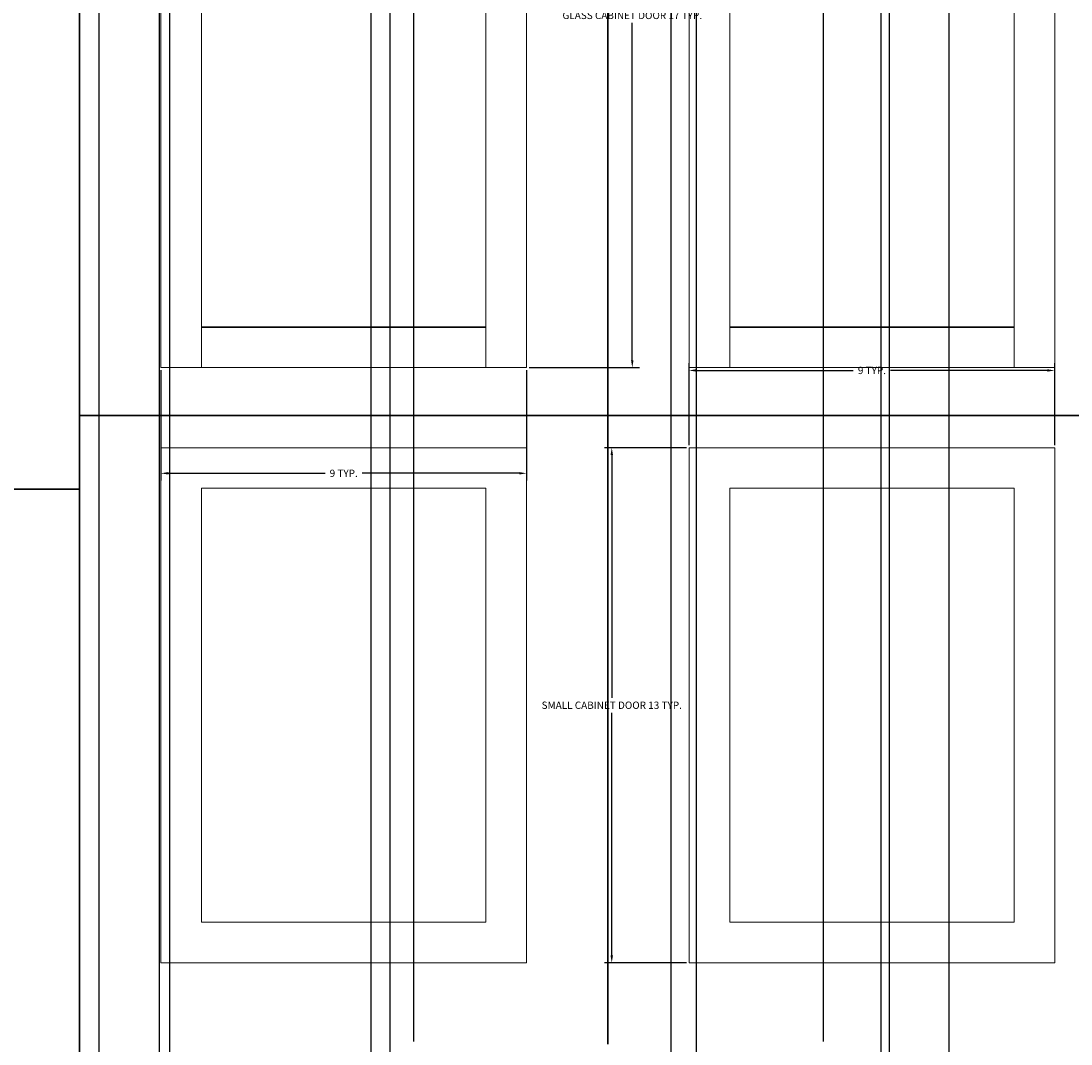
# Model space of a CAD drawing. Units: inches. Extents: x 27 to 200, y -50 to 102.
# Tile 19 of 26: x 119 to 145, y 52 to 77. Entities that reach past the tile are written whole.
import ezdxf

# ---------------------------------------------------------------- set-up
doc = ezdxf.new("R2010")
doc.units = ezdxf.units.IN
doc.header["$MEASUREMENT"] = 0
for name, color, linetype, lineweight in [('A-ANNO-DIMS', 2, 'Continuous', 18), ('A-ELEV', 7, 'Continuous', 35), ('A-FURN', 8, 'Continuous', 18)]:
    doc.layers.add(name, color=color, linetype=linetype, lineweight=lineweight)
doc.styles.get("Standard").update_dxf_attribs({"font": 'arial.ttf'})
doc.dimstyles.get("Standard").update_dxf_attribs({"dimtxt": 0.18, "dimasz": 0.18, "dimexe": 0.18, "dimexo": 0.0625, "dimgap": 0.09, "dimtad": 0, "dimtih": 1, "dimtoh": 1, "dimdec": 4, "dimzin": 0, "dimdsep": 46, "dimtxsty": 'Standard', "dimcen": 0.09, "dimadec": 0, "dimazin": 0, "dimtfac": 1, "dimtdec": 4, "dimtofl": 0, "dimtmove": 0, "dimatfit": 3, "dimfxl": 1, "dimtolj": 1, "dimtzin": 0, "dimarcsym": 0})

# ---------------------------------------------------------------- blocks, each defined once
blk = doc.blocks.new('CAB-DOOR-GLASS')
for p, q in [((0, 17.345), (9, 17.345)), ((0, 0), (0, 17.345)), ((9, 17.345), (9, 0)), ((1, 16.345), (8, 16.345)), ((1, 0), (1, 16.345)), ((8, 16.345), (8, 0)), ((9, 0), (0, 0))]:
    blk.add_line(p, q)
blk = doc.blocks.new('CAB-DOOR-SMALL')
for p, q in [((0, 0), (0, 12.683)), ((0, 12.683), (9, 12.683)), ((9, 12.683), (9, 0)), ((1, 1), (1, 11.683)), ((1, 11.683), (8, 11.683)), ((8, 11.683), (8, 1)), ((8, 1), (1, 1)), ((9, 0), (0, 0))]:
    blk.add_line(p, q)
blk = doc.blocks.new('*D9')
at = {"layer": 'A-ANNO-DIMS', "color": 0, "lineweight": -2, "transparency": 16777216}
for p, q in [((131.479, 85.926), (134.199, 85.926)), ((134.019, 85.746), (134.019, 77.437)), ((134.019, 68.761), (134.019, 77.071)), ((131.479, 68.581), (134.199, 68.581))]:
    blk.add_line(p, q, dxfattribs=at)
at = {"layer": 'A-ANNO-DIMS', "color": 0, "transparency": 16777216}
for points in [[(133.989, 85.746), (134.049, 85.746), (134.019, 85.926)], [(133.989, 68.761), (134.049, 68.761), (134.019, 68.581)]]:
    blk.add_solid(points, dxfattribs=at)
at = {"layer": 'Defpoints', "color": 0, "transparency": 16777216}
for p in [(131.417, 85.926), (134.019, 85.926), (131.417, 68.581)]:
    blk.add_point(p, dxfattribs=at)
at = {"layer": 'A-ANNO-DIMS', "color": 0, "transparency": 16777216, "insert": (134.019, 77.254), "char_height": 0.18, "attachment_point": 5}
blk.add_mtext('\\A1;GLASS CABINET DOOR 17 TYP.', dxfattribs=at)
blk = doc.blocks.new('*D10')
at = {"layer": 'A-ANNO-DIMS', "color": 0, "lineweight": -2, "transparency": 16777216}
for p, q in [((122.417, 68.519), (122.417, 65.799)), ((131.417, 68.519), (131.417, 65.799)), ((122.597, 65.979), (126.459, 65.979)), ((131.237, 65.979), (127.375, 65.979))]:
    blk.add_line(p, q, dxfattribs=at)
at = {"layer": 'A-ANNO-DIMS', "color": 0, "transparency": 16777216}
for points in [[(122.597, 66.009), (122.597, 65.949), (122.417, 65.979)], [(131.237, 66.009), (131.237, 65.949), (131.417, 65.979)]]:
    blk.add_solid(points, dxfattribs=at)
at = {"layer": 'Defpoints', "color": 0, "transparency": 16777216}
for p in [(122.417, 68.581), (131.417, 68.581), (131.417, 65.979)]:
    blk.add_point(p, dxfattribs=at)
at = {"layer": 'A-ANNO-DIMS', "color": 0, "transparency": 16777216, "insert": (126.917, 65.979), "char_height": 0.18, "attachment_point": 5}
blk.add_mtext('\\A1;9 TYP.', dxfattribs=at)
blk = doc.blocks.new('*D11')
at = {"layer": 'A-ANNO-DIMS', "color": 0, "lineweight": -2, "transparency": 16777216}
for p, q in [((135.354, 66.609), (133.334, 66.609)), ((133.514, 66.429), (133.514, 60.451)), ((133.514, 54.106), (133.514, 60.085)), ((135.354, 53.926), (133.334, 53.926))]:
    blk.add_line(p, q, dxfattribs=at)
at = {"layer": 'A-ANNO-DIMS', "color": 0, "transparency": 16777216}
for points in [[(133.484, 66.429), (133.544, 66.429), (133.514, 66.609)], [(133.484, 54.106), (133.544, 54.106), (133.514, 53.926)]]:
    blk.add_solid(points, dxfattribs=at)
at = {"layer": 'Defpoints', "color": 0, "transparency": 16777216}
for p in [(133.514, 66.609), (135.417, 66.609), (135.417, 53.926)]:
    blk.add_point(p, dxfattribs=at)
at = {"layer": 'A-ANNO-DIMS', "color": 0, "transparency": 16777216, "insert": (133.514, 60.268), "char_height": 0.18, "attachment_point": 5}
blk.add_mtext('\\A1;SMALL CABINET DOOR 13 TYP.', dxfattribs=at)
blk = doc.blocks.new('*D12')
at = {"layer": 'A-ANNO-DIMS', "color": 0, "lineweight": -2, "transparency": 16777216}
for p, q in [((135.417, 66.672), (135.417, 68.692)), ((135.597, 68.512), (139.459, 68.512)), ((144.237, 68.512), (140.375, 68.512)), ((144.417, 66.672), (144.417, 68.692))]:
    blk.add_line(p, q, dxfattribs=at)
at = {"layer": 'A-ANNO-DIMS', "color": 0, "transparency": 16777216}
for points in [[(135.597, 68.542), (135.597, 68.482), (135.417, 68.512)], [(144.237, 68.542), (144.237, 68.482), (144.417, 68.512)]]:
    blk.add_solid(points, dxfattribs=at)
at = {"layer": 'Defpoints', "color": 0, "transparency": 16777216}
for p in [(144.417, 68.512), (135.417, 66.609), (144.417, 66.609)]:
    blk.add_point(p, dxfattribs=at)
at = {"layer": 'A-ANNO-DIMS', "color": 0, "transparency": 16777216, "insert": (139.917, 68.512), "char_height": 0.18, "attachment_point": 5}
blk.add_mtext('\\A1;9 TYP.', dxfattribs=at)
blk = doc.blocks.new('*D49')
at = {"layer": 'A-ANNO-DIMS', "color": 0, "lineweight": -2, "transparency": 16777216}
for p, q in [((120.417, 51.989), (120.417, 102.306)), ((120.597, 102.126), (124.208, 102.126)), ((128.466, 102.126), (124.856, 102.126)), ((128.646, 51.989), (128.646, 102.306))]:
    blk.add_line(p, q, dxfattribs=at)
at = {"layer": 'A-ANNO-DIMS', "color": 0, "transparency": 16777216}
for points in [[(120.597, 102.156), (120.597, 102.096), (120.417, 102.126)], [(128.466, 102.156), (128.466, 102.096), (128.646, 102.126)]]:
    blk.add_solid(points, dxfattribs=at)
at = {"layer": 'Defpoints', "color": 0, "transparency": 16777216}
for p in [(128.646, 102.126), (120.417, 51.926), (128.646, 51.926)]:
    blk.add_point(p, dxfattribs=at)
at = {"layer": 'A-ANNO-DIMS', "color": 0, "transparency": 16777216, "insert": (124.532, 102.126), "char_height": 0.18, "attachment_point": 5}
blk.add_mtext('\\A1;8.23', dxfattribs=at)
blk = doc.blocks.new('*D50')
at = {"layer": 'A-ANNO-DIMS', "color": 0, "lineweight": -2, "transparency": 16777216}
for p, q in [((138.722, 51.989), (138.722, 102.306)), ((138.902, 102.126), (142.176, 102.126)), ((146.237, 102.126), (142.963, 102.126)), ((146.417, 51.989), (146.417, 102.306))]:
    blk.add_line(p, q, dxfattribs=at)
at = {"layer": 'A-ANNO-DIMS', "color": 0, "transparency": 16777216}
for points in [[(138.902, 102.156), (138.902, 102.096), (138.722, 102.126)], [(146.237, 102.156), (146.237, 102.096), (146.417, 102.126)]]:
    blk.add_solid(points, dxfattribs=at)
at = {"layer": 'Defpoints', "color": 0, "transparency": 16777216}
for p in [(146.417, 102.126), (138.722, 51.926), (146.417, 51.926)]:
    blk.add_point(p, dxfattribs=at)
at = {"layer": 'A-ANNO-DIMS', "color": 0, "transparency": 16777216, "insert": (142.569, 102.126), "char_height": 0.18, "attachment_point": 5}
blk.add_mtext('\\A1;7.695', dxfattribs=at)
blk = doc.blocks.new('*D53')
at = {"layer": 'A-ANNO-DIMS', "color": 0, "lineweight": -2, "transparency": 16777216}
for p, q in [((120.895, 14.04), (120.895, 102.306)), ((121.075, 102.126), (130.962, 102.126)), ((141.636, 102.126), (131.75, 102.126)), ((141.816, 14.04), (141.816, 102.306))]:
    blk.add_line(p, q, dxfattribs=at)
at = {"layer": 'A-ANNO-DIMS', "color": 0, "transparency": 16777216}
for points in [[(121.075, 102.156), (121.075, 102.096), (120.895, 102.126)], [(141.636, 102.156), (141.636, 102.096), (141.816, 102.126)]]:
    blk.add_solid(points, dxfattribs=at)
at = {"layer": 'Defpoints', "color": 0, "transparency": 16777216}
for p in [(141.816, 102.126), (120.895, 13.977), (141.816, 13.977)]:
    blk.add_point(p, dxfattribs=at)
at = {"layer": 'A-ANNO-DIMS', "color": 0, "transparency": 16777216, "insert": (131.356, 102.126), "char_height": 0.18, "attachment_point": 5}
blk.add_mtext('\\A1;20.92', dxfattribs=at)
blk = doc.blocks.new('*D57')
at = {"layer": 'A-ANNO-DIMS', "color": 0, "lineweight": -2, "transparency": 16777216}
for p, q in [((122.38, 4.48), (122.38, 102.306)), ((122.56, 102.126), (130.875, 102.126)), ((139.961, 102.126), (131.645, 102.126)), ((140.141, 4.48), (140.141, 102.306))]:
    blk.add_line(p, q, dxfattribs=at)
at = {"layer": 'A-ANNO-DIMS', "color": 0, "transparency": 16777216}
for points in [[(122.56, 102.156), (122.56, 102.096), (122.38, 102.126)], [(139.961, 102.156), (139.961, 102.096), (140.141, 102.126)]]:
    blk.add_solid(points, dxfattribs=at)
at = {"layer": 'Defpoints', "color": 0, "transparency": 16777216}
for p in [(140.141, 102.126), (122.38, 4.418), (140.141, 4.418)]:
    blk.add_point(p, dxfattribs=at)
at = {"layer": 'A-ANNO-DIMS', "color": 0, "transparency": 16777216, "insert": (131.26, 102.126), "char_height": 0.18, "attachment_point": 5}
blk.add_mtext('\\A1;17.76', dxfattribs=at)
blk = doc.blocks.new('*D59')
at = {"layer": 'A-ANNO-DIMS', "color": 0, "lineweight": -2, "transparency": 16777216}
for p, q in [((127.595, -0.162), (127.595, 102.306)), ((127.775, 102.126), (130.893, 102.126)), ((134.798, 102.126), (131.679, 102.126)), ((134.978, -0.162), (134.978, 102.306))]:
    blk.add_line(p, q, dxfattribs=at)
at = {"layer": 'A-ANNO-DIMS', "color": 0, "transparency": 16777216}
for points in [[(127.775, 102.156), (127.775, 102.096), (127.595, 102.126)], [(134.798, 102.156), (134.798, 102.096), (134.978, 102.126)]]:
    blk.add_solid(points, dxfattribs=at)
at = {"layer": 'Defpoints', "color": 0, "transparency": 16777216}
for p in [(134.978, 102.126), (127.595, -0.225), (134.978, -0.225)]:
    blk.add_point(p, dxfattribs=at)
at = {"layer": 'A-ANNO-DIMS', "color": 0, "transparency": 16777216, "insert": (131.286, 102.126), "char_height": 0.18, "attachment_point": 5}
blk.add_mtext('\\A1;7.383', dxfattribs=at)
blk = doc.blocks.new('*D61')
at = {"layer": 'A-ANNO-DIMS', "color": 0, "lineweight": -2, "transparency": 16777216}
for p, q in [((122.638, -4.237), (122.638, 102.306)), ((122.818, 102.126), (131.125, 102.126)), ((140.167, 102.126), (131.86, 102.126)), ((140.347, -4.237), (140.347, 102.306))]:
    blk.add_line(p, q, dxfattribs=at)
at = {"layer": 'A-ANNO-DIMS', "color": 0, "transparency": 16777216}
for points in [[(122.818, 102.156), (122.818, 102.096), (122.638, 102.126)], [(140.167, 102.156), (140.167, 102.096), (140.347, 102.126)]]:
    blk.add_solid(points, dxfattribs=at)
at = {"layer": 'Defpoints', "color": 0, "transparency": 16777216}
for p in [(140.347, 102.126), (122.638, -4.3), (140.347, -4.3)]:
    blk.add_point(p, dxfattribs=at)
at = {"layer": 'A-ANNO-DIMS', "color": 0, "transparency": 16777216, "insert": (131.493, 102.126), "char_height": 0.18, "attachment_point": 5}
blk.add_mtext('\\A1;17.71', dxfattribs=at)
blk = doc.blocks.new('*D63')
at = {"layer": 'A-ANNO-DIMS', "color": 0, "lineweight": -2, "transparency": 16777216}
for p, q in [((128.059, -9.034), (128.059, 102.306)), ((128.239, 102.126), (131.435, 102.126)), ((135.417, 102.126), (132.221, 102.126)), ((135.597, -9.034), (135.597, 102.306))]:
    blk.add_line(p, q, dxfattribs=at)
at = {"layer": 'A-ANNO-DIMS', "color": 0, "transparency": 16777216}
for points in [[(128.239, 102.156), (128.239, 102.096), (128.059, 102.126)], [(135.417, 102.156), (135.417, 102.096), (135.597, 102.126)]]:
    blk.add_solid(points, dxfattribs=at)
at = {"layer": 'Defpoints', "color": 0, "transparency": 16777216}
for p in [(135.597, 102.126), (128.059, -9.097), (135.597, -9.097)]:
    blk.add_point(p, dxfattribs=at)
at = {"layer": 'A-ANNO-DIMS', "color": 0, "transparency": 16777216, "insert": (131.828, 102.126), "char_height": 0.18, "attachment_point": 5}
blk.add_mtext('\\A1;7.538', dxfattribs=at)

msp = doc.modelspace()

# ---------------------------------------------------------------- linework, layer by layer
at = {"layer": 'A-ELEV'}
for p, q in [((120.4169, 87.9264), (120.4169, 51.9264)), ((133.4169, 87.9264), (133.4169, 51.9264)), ((130.4169, 69.5812), (123.4169, 69.5812)), ((143.4169, 69.5812), (136.4169, 69.5812)), ((120.4169, 67.3991), (146.4169, 67.3991)), ((84.4169, 65.5865), (120.4169, 65.5865))]:
    msp.add_line(p, q, dxfattribs=at)
msp.add_lwpolyline([(84.4169, 65.5865), (120.4169, 65.5865), (120.4169, 39.8559), (84.4169, 39.8559)], close=True, dxfattribs=at)

# ---------------------------------------------------------------- block references
at = {"layer": 'A-FURN'}
for name, p in [('CAB-DOOR-GLASS', (122.417, 68.581)), ('CAB-DOOR-GLASS', (135.417, 68.581)), ('CAB-DOOR-SMALL', (135.417, 53.926))]:
    msp.add_blockref(name, p, dxfattribs=at)
at = {"layer": 'A-FURN', "rotation": 180}
msp.add_blockref('CAB-DOOR-SMALL', (131.4168, 66.6096), dxfattribs=at)

# ---------------------------------------------------------------- dimensions: what is measured, and where the dimension line sits
at = {"layer": 'A-ANNO-DIMS'}
for base, p1, p2, override, picture, middle in [((128.6463, 102.1264), (120.4169, 51.9264), (128.6463, 51.9264), {"dimdec": 2, "dimlfac": 1, "dimrnd": 0, "dimzin": 0, "dimdsep": 46, "dimlunit": 2}, '*D49', (124.5316, 102.1264)), ((141.8163, 102.1264), (120.8954, 13.9773), (141.8163, 13.9773), {"dimdec": 2, "dimlfac": 1, "dimrnd": 0, "dimzin": 0, "dimdsep": 46, "dimlunit": 2}, '*D53', (131.3558, 102.1264)), ((140.1406, 102.1264), (122.38, 4.4177), (140.1406, 4.4177), {"dimdec": 2, "dimlfac": 1, "dimrnd": 0, "dimzin": 0, "dimdsep": 46, "dimlunit": 2}, '*D57', (131.2603, 102.1264)), ((140.3471, 102.1264), (122.6381, -4.2997), (140.3471, -4.2997), {"dimdec": 2, "dimlfac": 1, "dimrnd": 0, "dimzin": 0, "dimdsep": 46, "dimlunit": 2}, '*D61', (131.4926, 102.1264)), ((134.9776, 102.1264), (127.5946, -0.2247), (134.9776, -0.2247), {"dimdec": 3, "dimlfac": 1, "dimrnd": 0, "dimzin": 0, "dimdsep": 46, "dimlunit": 2}, '*D59', (131.2861, 102.1264)), ((135.5972, 102.1264), (128.0592, -9.0968), (135.5972, -9.0968), {"dimdec": 3, "dimlfac": 1, "dimrnd": 0, "dimzin": 0, "dimdsep": 46, "dimlunit": 2}, '*D63', (131.8282, 102.1264)), ((146.4169, 102.1264), (138.7218, 51.9264), (146.4169, 51.9264), {"dimdec": 3, "dimlfac": 1, "dimrnd": 0, "dimzin": 0, "dimdsep": 46, "dimlunit": 2}, '*D50', (142.5694, 102.1264))]:
    dim = msp.add_linear_dim(base=base, p1=p1, p2=p2, dimstyle='Standard', override=override, dxfattribs=at)
    dim.commit()
    dim.dimension.update_dxf_attribs({"geometry": picture, "text_midpoint": middle})
for base, p1, p2, text, picture, middle in [((134.0187, 85.9264), (131.4169, 68.5812), (131.4169, 85.9264), 'GLASS CABINET DOOR <> TYP.', '*D9', (134.0187, 77.2538)), ((133.5145, 66.6092), (135.4169, 53.9264), (135.4169, 66.6092), 'SMALL CABINET DOOR <> TYP.', '*D11', (133.5145, 60.2678))]:
    dim = msp.add_linear_dim(base=base, p1=p1, p2=p2, angle=90, text=text, dimstyle='Standard', override={"dimdec": 0, "dimrnd": 0, "dimzin": 0, "dimlunit": 2}, dxfattribs=at)
    dim.commit()
    dim.dimension.update_dxf_attribs({"geometry": picture, "text_midpoint": middle})
for base, p1, p2, picture, middle in [((144.4169, 68.5116), (135.4169, 66.6092), (144.4169, 66.6092), '*D12', (139.9169, 68.5116)), ((131.4169, 65.9794), (122.4169, 68.5812), (131.4169, 68.5812), '*D10', (126.9169, 65.9794))]:
    dim = msp.add_linear_dim(base=base, p1=p1, p2=p2, text='<> TYP.', dimstyle='Standard', override={"dimdec": 0, "dimrnd": 0, "dimzin": 0, "dimlunit": 2}, dxfattribs=at)
    dim.commit()
    dim.dimension.update_dxf_attribs({"geometry": picture, "text_midpoint": middle})

doc.saveas('drawing.dxf')
